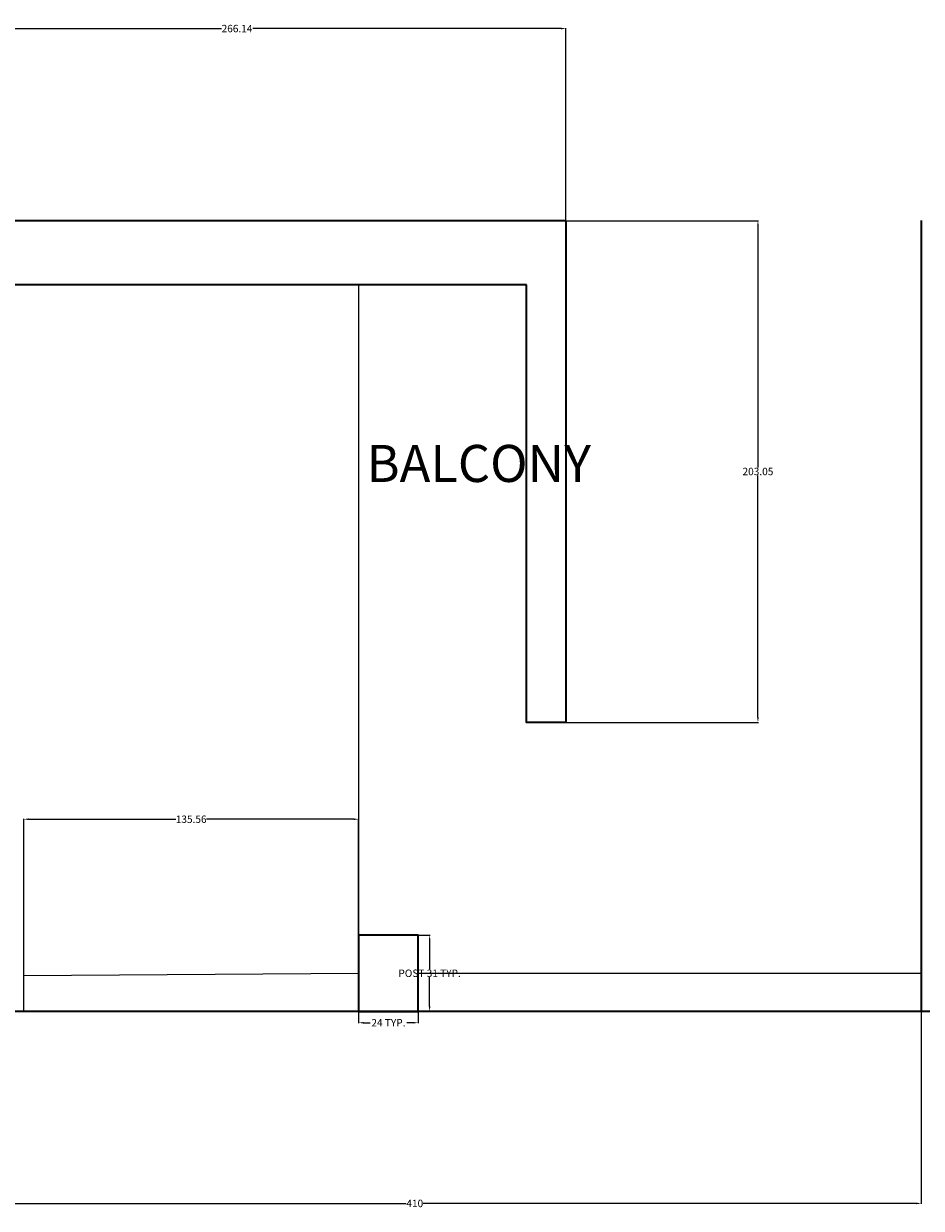
# Model space of a CAD drawing. Units: centimetres. Extents: x -121 to 3851, y -16 to 1180.
# Tile 11 of 16: x 2458 to 2821, y 16 to 495. Entities that reach past the tile are written whole.
import ezdxf

# ---------------------------------------------------------------- set-up
doc = ezdxf.new("R2010")
doc.units = ezdxf.units.CM
doc.header["$MEASUREMENT"] = 0
for name, color, linetype, lineweight in [('A-ANNO-DIMS', 2, 'Continuous', 18), ('A-AREA-IDEN', 3, 'Continuous', 18), ('A-COLS', 7, 'Continuous', 35), ('A-FLOR', 8, 'Continuous', 25), ('A-FLOR-HRAL', 4, 'Continuous', 18), ('A-WALL', 7, 'Continuous', 35)]:
    doc.layers.add(name, color=color, linetype=linetype, lineweight=lineweight)
doc.styles.get("Standard").update_dxf_attribs({"font": 'arial.ttf'})
doc.dimstyles.get("Standard").update_dxf_attribs({"dimtxt": 3, "dimasz": 2, "dimexe": 0.18, "dimexo": 0.0625, "dimgap": 0.09, "dimtad": 0, "dimtih": 1, "dimtoh": 1, "dimdec": 0, "dimzin": 0, "dimdsep": 46, "dimtxsty": 'Standard', "dimcen": 0.09, "dimadec": 0, "dimazin": 0, "dimtfac": 1, "dimtdec": 0, "dimtofl": 0, "dimtmove": 0, "dimatfit": 3, "dimfxl": 1, "dimtolj": 1, "dimtzin": 0, "dimarcsym": 0})

# ---------------------------------------------------------------- blocks, each defined once
blk = doc.blocks.new('POST-24X31CM')
blk.add_lwpolyline([(0, 0), (24.1, 0), (24.1, 30.82), (0, 30.82)], close=True)
blk = doc.blocks.new('*D35')
at = {"layer": 'A-ANNO-DIMS', "color": 0, "lineweight": -2, "transparency": 16777216}
for p, q in [((2617.71, 126.54), (2622.45, 126.54)), ((2622.27, 124.54), (2622.27, 112.77)), ((2622.27, 97.72), (2622.27, 109.49)), ((2617.71, 95.72), (2622.45, 95.72))]:
    blk.add_line(p, q, dxfattribs=at)
at = {"layer": 'A-ANNO-DIMS', "color": 0, "transparency": 16777216}
for points in [[(2621.94, 124.54), (2622.61, 124.54), (2622.27, 126.54)], [(2621.94, 97.72), (2622.61, 97.72), (2622.27, 95.72)]]:
    blk.add_solid(points, dxfattribs=at)
at = {"layer": 'Defpoints', "color": 0, "transparency": 16777216}
for p in [(2617.65, 126.54), (2622.27, 126.54), (2617.65, 95.72)]:
    blk.add_point(p, dxfattribs=at)
at = {"layer": 'A-ANNO-DIMS', "color": 0, "transparency": 16777216, "insert": (2622.27, 111.13), "char_height": 3, "attachment_point": 5}
blk.add_mtext('\\A1;POST 31 TYP.', dxfattribs=at)
blk = doc.blocks.new('*D36')
at = {"layer": 'A-ANNO-DIMS', "color": 0, "lineweight": -2, "transparency": 16777216}
for p, q in [((2593.55, 95.66), (2593.55, 90.92)), ((2595.55, 91.1), (2598.18, 91.1)), ((2615.65, 91.1), (2613.02, 91.1)), ((2617.65, 95.66), (2617.65, 90.92))]:
    blk.add_line(p, q, dxfattribs=at)
at = {"layer": 'A-ANNO-DIMS', "color": 0, "transparency": 16777216}
for points in [[(2595.55, 91.43), (2595.55, 90.77), (2593.55, 91.1)], [(2615.65, 91.43), (2615.65, 90.77), (2617.65, 91.1)]]:
    blk.add_solid(points, dxfattribs=at)
at = {"layer": 'Defpoints', "color": 0, "transparency": 16777216}
for p in [(2593.55, 95.72), (2617.65, 95.72), (2617.65, 91.1)]:
    blk.add_point(p, dxfattribs=at)
at = {"layer": 'A-ANNO-DIMS', "color": 0, "transparency": 16777216, "insert": (2605.6, 91.1), "char_height": 3, "attachment_point": 5}
blk.add_mtext('\\A1;24 TYP.', dxfattribs=at)
blk = doc.blocks.new('*D67')
at = {"layer": 'A-ANNO-DIMS', "color": 0, "lineweight": -2, "transparency": 16777216}
for p, q in [((2411.26, 95.66), (2411.26, 17.79)), ((2821.26, 95.66), (2821.26, 17.79)), ((2413.26, 17.97), (2612.8, 17.97)), ((2819.26, 17.97), (2619.72, 17.97))]:
    blk.add_line(p, q, dxfattribs=at)
at = {"layer": 'A-ANNO-DIMS', "color": 0, "transparency": 16777216}
for points in [[(2413.26, 18.31), (2413.26, 17.64), (2411.26, 17.97)], [(2819.26, 18.31), (2819.26, 17.64), (2821.26, 17.97)]]:
    blk.add_solid(points, dxfattribs=at)
at = {"layer": 'Defpoints', "color": 0, "transparency": 16777216}
for p in [(2411.26, 95.72), (2821.26, 95.72), (2821.26, 17.97)]:
    blk.add_point(p, dxfattribs=at)
at = {"layer": 'A-ANNO-DIMS', "color": 0, "transparency": 16777216, "insert": (2616.26, 17.97), "char_height": 3, "attachment_point": 5}
blk.add_mtext('\\A1;410', dxfattribs=at)
blk = doc.blocks.new('*D76')
at = {"layer": 'A-ANNO-DIMS', "color": 0, "lineweight": -2, "transparency": 16777216}
for p, q in [((2457.99, 95.79), (2457.99, 173.65)), ((2459.99, 173.47), (2519.59, 173.47)), ((2591.55, 173.47), (2531.94, 173.47)), ((2593.55, 95.79), (2593.55, 173.65))]:
    blk.add_line(p, q, dxfattribs=at)
at = {"layer": 'A-ANNO-DIMS', "color": 0, "transparency": 16777216}
for points in [[(2459.99, 173.81), (2459.99, 173.14), (2457.99, 173.47)], [(2591.55, 173.81), (2591.55, 173.14), (2593.55, 173.47)]]:
    blk.add_solid(points, dxfattribs=at)
at = {"layer": 'Defpoints', "color": 0, "transparency": 16777216}
for p in [(2593.55, 173.47), (2457.99, 95.72), (2593.55, 95.72)]:
    blk.add_point(p, dxfattribs=at)
at = {"layer": 'A-ANNO-DIMS', "color": 0, "transparency": 16777216, "insert": (2525.77, 173.47), "char_height": 3, "attachment_point": 5}
blk.add_mtext('\\A1;135.56', dxfattribs=at)
blk = doc.blocks.new('*D78')
at = {"layer": 'A-ANNO-DIMS', "color": 0, "lineweight": -2, "transparency": 16777216}
for p, q in [((2411.26, 415.79), (2411.26, 493.65)), ((2413.26, 493.47), (2538, 493.47)), ((2675.4, 493.47), (2550.67, 493.47)), ((2677.4, 415.79), (2677.4, 493.65))]:
    blk.add_line(p, q, dxfattribs=at)
at = {"layer": 'A-ANNO-DIMS', "color": 0, "transparency": 16777216}
for points in [[(2413.26, 493.81), (2413.26, 493.14), (2411.26, 493.47)], [(2675.4, 493.81), (2675.4, 493.14), (2677.4, 493.47)]]:
    blk.add_solid(points, dxfattribs=at)
at = {"layer": 'Defpoints', "color": 0, "transparency": 16777216}
for p in [(2677.4, 493.47), (2411.26, 415.72), (2677.4, 415.72)]:
    blk.add_point(p, dxfattribs=at)
at = {"layer": 'A-ANNO-DIMS', "color": 0, "transparency": 16777216, "insert": (2544.33, 493.47), "char_height": 3, "attachment_point": 5}
blk.add_mtext('\\A1;266.14', dxfattribs=at)
blk = doc.blocks.new('*D79')
at = {"layer": 'A-ANNO-DIMS', "color": 0, "lineweight": -2, "transparency": 16777216}
for p, q in [((2677.46, 415.72), (2755.33, 415.72)), ((2755.15, 413.72), (2755.15, 315.82)), ((2755.15, 214.67), (2755.15, 312.58)), ((2677.46, 212.67), (2755.33, 212.67))]:
    blk.add_line(p, q, dxfattribs=at)
at = {"layer": 'A-ANNO-DIMS', "color": 0, "transparency": 16777216}
for points in [[(2754.82, 413.72), (2755.48, 413.72), (2755.15, 415.72)], [(2754.82, 214.67), (2755.48, 214.67), (2755.15, 212.67)]]:
    blk.add_solid(points, dxfattribs=at)
at = {"layer": 'Defpoints', "color": 0, "transparency": 16777216}
for p in [(2677.4, 415.72), (2677.4, 212.67), (2755.15, 212.67)]:
    blk.add_point(p, dxfattribs=at)
at = {"layer": 'A-ANNO-DIMS', "color": 0, "transparency": 16777216, "insert": (2755.15, 314.2), "char_height": 3, "attachment_point": 5}
blk.add_mtext('\\A1;203.05', dxfattribs=at)

msp = doc.modelspace()

# ---------------------------------------------------------------- linework, layer by layer
at = {"layer": 'A-FLOR'}
msp.add_line((2593.5502, 389.7228), (2593.5502, 95.7228), dxfattribs=at)
at = {"layer": 'A-FLOR-HRAL'}
for p, q in [((2457.9883, 110.2005), (2593.5502, 111.1316)), ((2617.6503, 111.1316), (2821.2642, 111.1316))]:
    msp.add_line(p, q, dxfattribs=at)
at = {"layer": 'A-WALL'}
for p, q in [((2411.2642, 415.7228), (2677.3995, 415.7228)), ((2821.2642, 415.7228), (2821.2642, 95.7228)), ((2661.5376, 389.7228), (2411.2642, 389.7228)), ((3767.2642, 95.7228), (2411.2642, 95.7228))]:
    msp.add_line(p, q, dxfattribs=at)
msp.add_lwpolyline([(2677.3995, 415.7228), (2677.3995, 212.6732), (2661.5376, 212.6732), (2661.5376, 389.7228)], dxfattribs=at)

# ---------------------------------------------------------------- block references
at = {"layer": 'A-COLS'}
msp.add_blockref('POST-24X31CM', (2593.55, 95.7227), dxfattribs=at)

# ---------------------------------------------------------------- texts
at = {"layer": 'A-AREA-IDEN', "insert": (2596.6993, 324.9688), "char_height": 15, "attachment_point": 1}
msp.add_mtext_dynamic_manual_height_columns('BALCONY', width=99.479102, gutter_width=1, heights=[0], dxfattribs=at)

# ---------------------------------------------------------------- dimensions: what is measured, and where the dimension line sits
at = {"layer": 'A-ANNO-DIMS'}
for base, p1, p2, override, picture, middle in [((2677.3995, 493.4728), (2411.2642, 415.7228), (2677.3995, 415.7228), {"dimdec": 2, "dimlfac": 1, "dimrnd": 0, "dimzin": 0, "dimdsep": 46, "dimlunit": 2}, '*D78', (2544.3319, 493.4728)), ((2593.5502, 173.4728), (2457.9883, 95.7228), (2593.5502, 95.7228), {"dimdec": 2, "dimlfac": 1, "dimrnd": 0, "dimzin": 0, "dimdsep": 46, "dimlunit": 2}, '*D76', (2525.7693, 173.4728)), ((2821.2642, 17.9728), (2411.2642, 95.7228), (2821.2642, 95.7228), {"dimdec": 0, "dimlfac": 1, "dimrnd": 0, "dimzin": 0, "dimdsep": 46, "dimlunit": 2}, '*D67', (2616.2642, 17.9728))]:
    dim = msp.add_linear_dim(base=base, p1=p1, p2=p2, dimstyle='Standard', override=override, dxfattribs=at)
    dim.commit()
    dim.dimension.update_dxf_attribs({"geometry": picture, "text_midpoint": middle})
dim = msp.add_linear_dim(base=(2755.1495, 212.6732), p1=(2677.3995, 415.7228), p2=(2677.3995, 212.6732), angle=270, dimstyle='Standard', override={"dimdec": 2, "dimlfac": 1, "dimrnd": 0, "dimzin": 0, "dimdsep": 46, "dimlunit": 2}, dxfattribs=at)
dim.commit()
dim.dimension.update_dxf_attribs({"geometry": '*D79', "text_midpoint": (2755.1495, 314.198)})
dim = msp.add_linear_dim(base=(2622.2729, 126.5403), p1=(2617.6503, 95.7228), p2=(2617.6503, 126.5403), angle=90, text='POST <> TYP.', dimstyle='Standard', override={"dimdec": 0, "dimlfac": 1, "dimrnd": 0, "dimzin": 0, "dimdsep": 46, "dimlunit": 2}, dxfattribs=at)
dim.commit()
dim.dimension.update_dxf_attribs({"geometry": '*D35', "text_midpoint": (2622.2729, 111.1316)})
dim = msp.add_linear_dim(base=(2617.6503, 91.1002), p1=(2593.5502, 95.7228), p2=(2617.6503, 95.7228), text='<> TYP.', dimstyle='Standard', override={"dimdec": 0, "dimlfac": 1, "dimrnd": 0, "dimzin": 0, "dimdsep": 46, "dimlunit": 2}, dxfattribs=at)
dim.commit()
dim.dimension.update_dxf_attribs({"geometry": '*D36', "text_midpoint": (2605.6002, 91.1002)})

doc.saveas('drawing.dxf')
